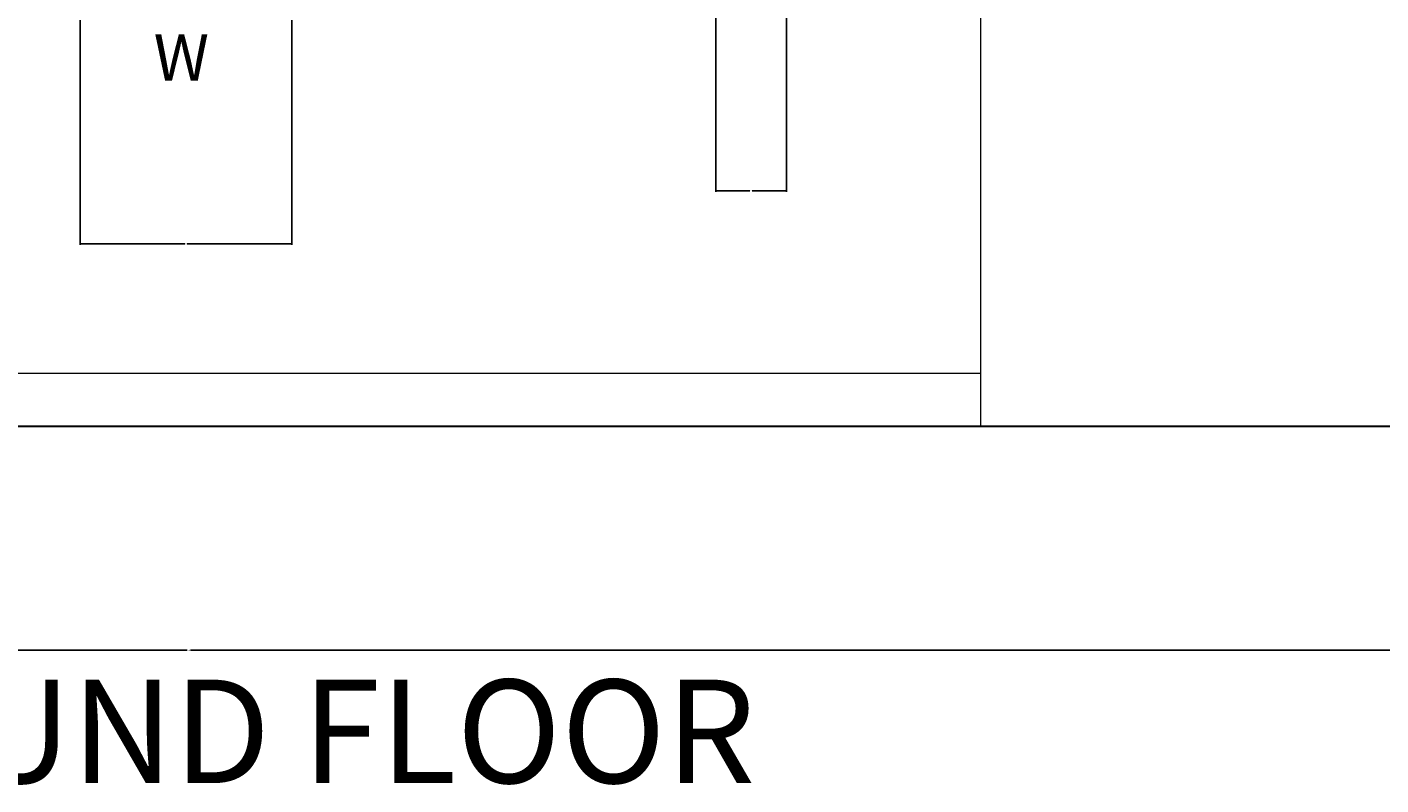
# Model space of a CAD drawing. Units: feet. Extents: x 2219 to 3039, y 1768 to 2369.
# Tile 3 of 16: x 2601 to 2831, y 1768 to 1897. Entities that reach past the tile are written whole.
import ezdxf

# ---------------------------------------------------------------- set-up
doc = ezdxf.new("R2010")
doc.units = ezdxf.units.FT
for name, color, linetype, lineweight in [('A-ANNO-DIMS', 2, 'Continuous', 18), ('A-ANNO-TEXT', 7, 'Continuous', 18), ('A-ANNO-TITL', 7, 'Continuous', 35), ('C-PROP', 7, 'Continuous', 30), ('C-SITE', 3, 'Continuous', 20)]:
    doc.layers.add(name, color=color, linetype=linetype, lineweight=lineweight)
doc.styles.get("Standard").update_dxf_attribs({"font": 'arial.ttf'})
doc.dimstyles.get("Standard").update_dxf_attribs({"dimtxt": 0.18, "dimasz": 0.18, "dimexe": 0.18, "dimexo": 0.0625, "dimgap": 0.09, "dimtad": 0, "dimtih": 1, "dimtoh": 1, "dimdec": 4, "dimzin": 0, "dimdsep": 46, "dimtxsty": 'Standard', "dimcen": 0.09, "dimadec": 0, "dimazin": 0, "dimtfac": 1, "dimtdec": 4, "dimtofl": 0, "dimtmove": 0, "dimatfit": 3, "dimfxl": 1, "dimtolj": 1, "dimtzin": 0, "dimarcsym": 0})

# ---------------------------------------------------------------- blocks, each defined once
blk = doc.blocks.new('*D46')
at = {"layer": 'A-ANNO-DIMS', "color": 0, "lineweight": -2, "transparency": 16777216}
for p, q in [((2257.4, 1828.86), (2257.4, 1790.69)), ((3000.4, 1828.86), (3000.4, 1790.69)), ((2257.58, 1790.87), (2628.61, 1790.87)), ((3000.22, 1790.87), (2629.19, 1790.87))]:
    blk.add_line(p, q, dxfattribs=at)
at = {"layer": 'A-ANNO-DIMS', "color": 0, "transparency": 16777216}
for points in [[(2257.58, 1790.9), (2257.58, 1790.84), (2257.4, 1790.87)], [(3000.22, 1790.9), (3000.22, 1790.84), (3000.4, 1790.87)]]:
    blk.add_solid(points, dxfattribs=at)
at = {"layer": 'Defpoints', "color": 0, "transparency": 16777216}
for p in [(2257.4, 1828.92), (3000.4, 1828.92), (3000.4, 1790.87)]:
    blk.add_point(p, dxfattribs=at)
at = {"layer": 'A-ANNO-DIMS', "color": 0, "transparency": 16777216, "insert": (2628.9, 1790.87), "char_height": 0.18, "attachment_point": 5}
blk.add_mtext('\\A1;743', dxfattribs=at)
blk = doc.blocks.new('*D62')
at = {"layer": 'A-ANNO-DIMS', "color": 0, "lineweight": -2, "transparency": 16777216}
for p, q in [((2610.4, 1897.86), (2610.4, 1859.69)), ((2646.4, 1897.86), (2646.4, 1859.69)), ((2610.58, 1859.87), (2628.18, 1859.87)), ((2646.22, 1859.87), (2628.62, 1859.87))]:
    blk.add_line(p, q, dxfattribs=at)
at = {"layer": 'A-ANNO-DIMS', "color": 0, "transparency": 16777216}
for points in [[(2610.58, 1859.9), (2610.58, 1859.84), (2610.4, 1859.87)], [(2646.22, 1859.9), (2646.22, 1859.84), (2646.4, 1859.87)]]:
    blk.add_solid(points, dxfattribs=at)
at = {"layer": 'Defpoints', "color": 0, "transparency": 16777216}
for p in [(2610.4, 1897.92), (2646.4, 1897.92), (2610.4, 1859.87)]:
    blk.add_point(p, dxfattribs=at)
at = {"layer": 'A-ANNO-DIMS', "color": 0, "transparency": 16777216, "insert": (2628.4, 1859.87), "char_height": 0.18, "attachment_point": 5}
blk.add_mtext('\\A1;36', dxfattribs=at)
blk = doc.blocks.new('*D63')
at = {"layer": 'A-ANNO-DIMS', "color": 0, "lineweight": -2, "transparency": 16777216}
for p, q in [((2718.4, 1906.86), (2718.4, 1868.69)), ((2730.4, 1906.86), (2730.4, 1868.69)), ((2718.58, 1868.87), (2724.19, 1868.87)), ((2730.22, 1868.87), (2724.61, 1868.87))]:
    blk.add_line(p, q, dxfattribs=at)
at = {"layer": 'A-ANNO-DIMS', "color": 0, "transparency": 16777216}
for points in [[(2718.58, 1868.9), (2718.58, 1868.84), (2718.4, 1868.87)], [(2730.22, 1868.9), (2730.22, 1868.84), (2730.4, 1868.87)]]:
    blk.add_solid(points, dxfattribs=at)
at = {"layer": 'Defpoints', "color": 0, "transparency": 16777216}
for p in [(2718.4, 1906.92), (2730.4, 1906.92), (2718.4, 1868.87)]:
    blk.add_point(p, dxfattribs=at)
at = {"layer": 'A-ANNO-DIMS', "color": 0, "transparency": 16777216, "insert": (2724.4, 1868.87), "char_height": 0.18, "attachment_point": 5}
blk.add_mtext('\\A1;12', dxfattribs=at)

msp = doc.modelspace()

# ---------------------------------------------------------------- linework, layer by layer
at = {"layer": 'C-PROP'}
msp.add_line((2314.4, 1828.923), (3000.4, 1828.923), dxfattribs=at)
at = {"layer": 'C-SITE'}
for p, q in [((2763.4, 1906.923), (2763.4, 1828.923)), ((2314.4, 1837.923), (2763.4, 1837.923))]:
    msp.add_line(p, q, dxfattribs=at)

# ---------------------------------------------------------------- texts
at = {"layer": 'A-ANNO-TEXT'}
msp.add_text('W', height=7.858, dxfattribs=at).set_placement((2622.902, 1887.6))
at = {"layer": 'A-ANNO-TITL'}
msp.add_text('GROUND FLOOR', height=17.56585, dxfattribs=at).set_placement((2542.155, 1768.289))

# ---------------------------------------------------------------- dimensions: what is measured, and where the dimension line sits
at = {"layer": 'A-ANNO-DIMS'}
for base, p1, p2, picture, middle in [((2718.4, 1868.873), (2730.4, 1906.923), (2718.4, 1906.923), '*D63', (2724.4, 1868.873)), ((2610.4, 1859.873), (2646.4, 1897.923), (2610.4, 1897.923), '*D62', (2628.4, 1859.873))]:
    dim = msp.add_linear_dim(base=base, p1=p1, p2=p2, angle=180, dimstyle='Standard', override={"dimdec": 0, "dimlfac": 1, "dimrnd": 0, "dimzin": 0, "dimdsep": 46, "dimlunit": 2}, dxfattribs=at)
    dim.commit()
    dim.dimension.update_dxf_attribs({"geometry": picture, "text_midpoint": middle})
dim = msp.add_linear_dim(base=(3000.4, 1790.873), p1=(2257.4, 1828.923), p2=(3000.4, 1828.923), dimstyle='Standard', override={"dimdec": 0, "dimlfac": 1, "dimrnd": 0, "dimzin": 0, "dimdsep": 46, "dimlunit": 2}, dxfattribs=at)
dim.commit()
dim.dimension.update_dxf_attribs({"geometry": '*D46', "text_midpoint": (2628.9, 1790.873)})

doc.saveas('drawing.dxf')
